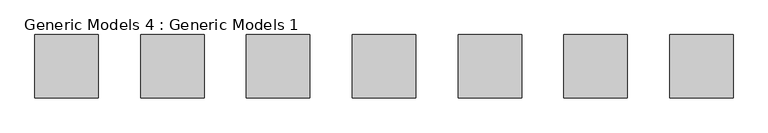
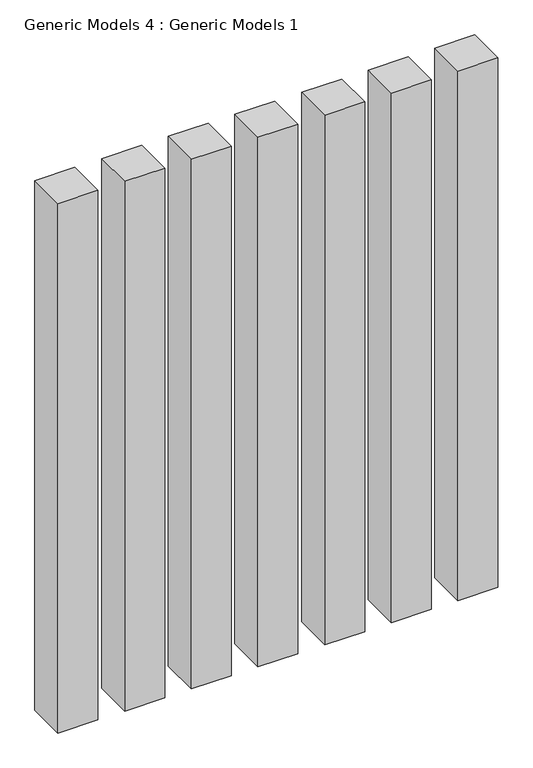
"""IFC4 building model written with IfcOpenShell, lengths in millimetres: proxy geometry, Generic Models 4 : Generic Models 1."""

from ifc_helpers import new_model, si_unit, origin, origin_with_axes, place, context, project, spatial, polyline, outline, extrude, source, transform, mapped, element, save


def generic_models_4_generic_models_1_81c75abe(model_context):
    return source(origin(), model_context, "Body", "SweptSolid", [
        extrude(outline(polyline([(-7673.9453682, 12607.034892), (-7673.9453682, 12378.434892), (-7902.5453682, 12378.434892), (-7902.5453682, 12607.034892), (-7673.9453682, 12607.034892)])), origin_with_axes(), (0.0, 0.0, 1.0), 3200.4),
        extrude(outline(polyline([(-7292.9453682, 12607.034892), (-7292.9453682, 12378.434892), (-7521.5453682, 12378.434892), (-7521.5453682, 12607.034892), (-7292.9453682, 12607.034892)])), origin_with_axes(), (0.0, 0.0, 1.0), 3200.4),
        extrude(outline(polyline([(-6911.9453682, 12607.034892), (-6911.9453682, 12378.434892), (-7140.5453682, 12378.434892), (-7140.5453682, 12607.034892), (-6911.9453682, 12607.034892)])), origin_with_axes(), (0.0, 0.0, 1.0), 3200.4),
        extrude(outline(polyline([(-6530.9453682, 12607.034892), (-6530.9453682, 12378.434892), (-6759.5453682, 12378.434892), (-6759.5453682, 12607.034892), (-6530.9453682, 12607.034892)])), origin_with_axes(), (0.0, 0.0, 1.0), 3200.4),
        extrude(outline(polyline([(-6149.9453682, 12607.034892), (-6149.9453682, 12378.434892), (-6378.5453682, 12378.434892), (-6378.5453682, 12607.034892), (-6149.9453682, 12607.034892)])), origin_with_axes(), (0.0, 0.0, 1.0), 3200.4),
        extrude(outline(polyline([(-5768.9453682, 12607.034892), (-5768.9453682, 12378.434892), (-5997.5453682, 12378.434892), (-5997.5453682, 12607.034892), (-5768.9453682, 12607.034892)])), origin_with_axes(), (0.0, 0.0, 1.0), 3200.4),
        extrude(outline(polyline([(-5387.9453682, 12607.034892), (-5387.9453682, 12378.434892), (-5616.5453682, 12378.434892), (-5616.5453682, 12607.034892), (-5387.9453682, 12607.034892)])), origin_with_axes(), (0.0, 0.0, 1.0), 3200.4),
    ])


if __name__ == "__main__":
    model = new_model("IFC4")
    model_context = context("Model", 3, world=origin())
    ifc_project = project(units=[si_unit("LENGTHUNIT", "METRE", prefix="MILLI")], contexts=[model_context])
    site = spatial("IfcSite", under=ifc_project)
    building = spatial("IfcBuilding", under=site)
    placement = place(None, origin())
    generic_models_4_generic_models_1_shape = generic_models_4_generic_models_1_81c75abe(model_context)
    element("IfcBuildingElementProxy", 1, Name="Generic Models 4 : Generic Models 1", ObjectType="Generic Models 4 : Generic Models 1", at=placement, inside=building, context=model_context, shape_type="MappedRepresentation", body=[
        mapped(generic_models_4_generic_models_1_shape, transform((0.0, 0.0, 0.0), x_axis=(1.0, 0.0, 0.0), y_axis=(0.0, 1.0, 0.0), z_axis=(0.0, 0.0, 1.0))),
    ])
    save(model, "model.ifc")

# Revit data of these elements
# Element 1 (IfcBuildingElementProxy, "Generic Models 4 : Generic Models 1")
#   Materials on its faces: "0 olive green"
# Materials
#   "0 olive green": class "Generic", colour RGB 120 120 120, transparency 0, Cost = 0
